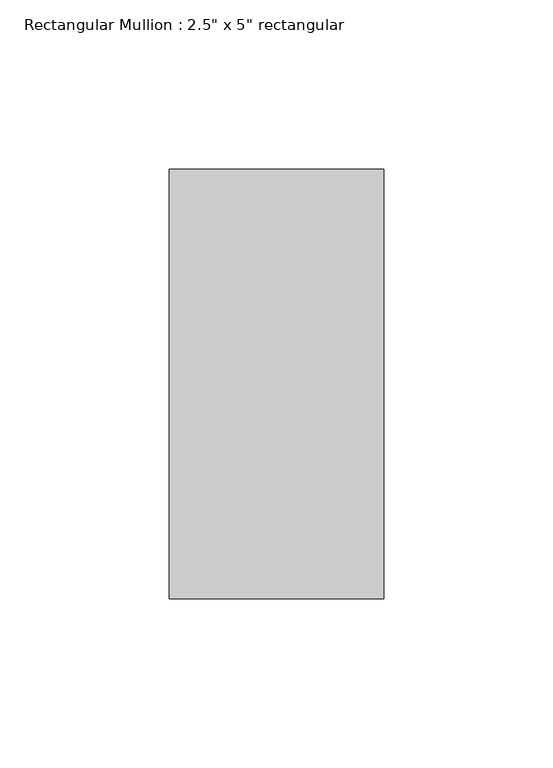
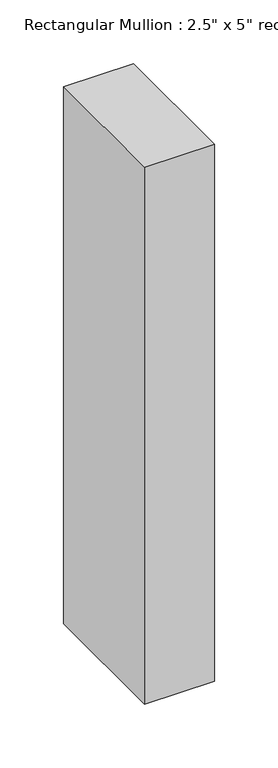
"""IFC4 building model written with IfcOpenShell, lengths in millimetres: member geometry."""

from ifc_helpers import new_model, si_unit, frame, origin, place, context, project, spatial, polyline, outline, extrude, source, transform, mapped, element, save


def member_0b7646a3(model_context):
    return source(origin(), model_context, "Body", "SweptSolid", [
        extrude(outline(polyline([(0.0, 63.5), (0.0, -63.5), (-63.5, -63.5), (-63.5, 63.5), (0.0, 63.5)])), frame((0.0, 0.0, -514.35), z_axis=(0.0, 0.0, 1.0), x_axis=(1.0, 0.0, 0.0)), (0.0, 0.0, 1.0), 514.35),
    ])


if __name__ == "__main__":
    model = new_model("IFC4")
    model_context = context("Model", 3, world=origin())
    ifc_project = project(units=[si_unit("LENGTHUNIT", "METRE", prefix="MILLI")], contexts=[model_context])
    site = spatial("IfcSite", under=ifc_project)
    building = spatial("IfcBuilding", under=site)
    placement = place(None, origin())
    member_shape = member_0b7646a3(model_context)
    element("IfcMember", 1, ObjectType="Rectangular Mullion : 2.5\" x 5\" rectangular", at=placement, inside=building, context=model_context, shape_type="MappedRepresentation", body=[
        mapped(member_shape, transform((0.0, 0.0, 0.0), x_axis=(1.0, 0.0, 0.0), y_axis=(0.0, 1.0, 0.0), z_axis=(0.0, 0.0, 1.0))),
    ])
    save(model, "model.ifc")

# Revit data of these elements
# Type "Rectangular Mullion : 2.5\" x 5\" rectangular"
#   built-in parameter 1007304 = 0.416667 (stored number, unit not read)
#   built-in parameter 1007301 = 0.104167 (stored number, unit not read)
#   built-in parameter 1007300 = 0.104167 (stored number, unit not read)
# Element 1 (IfcMember, "Rectangular Mullion : 2.5\" x 5\" rectangular")
#   Materials on its faces: "door black"
# Materials
#   "door black": class "Generic", colour RGB 120 120 120, transparency 0, Cost = 0
